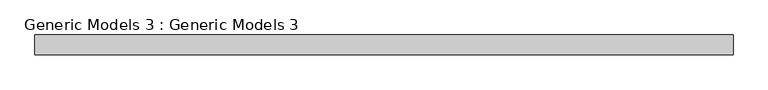
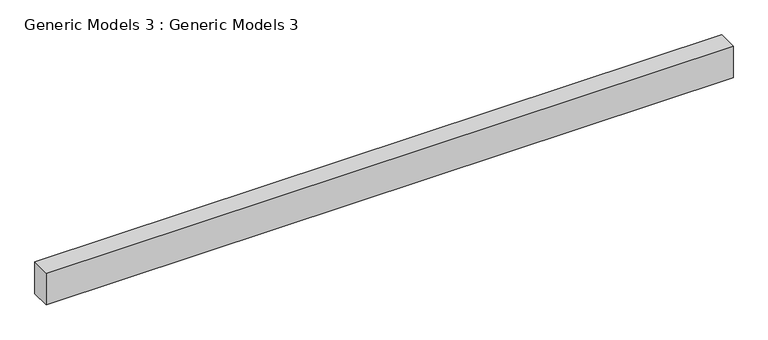
"""IFC4 building model written with IfcOpenShell, lengths in millimetres: proxy geometry, Generic Models 3 : Generic Models 3."""

from ifc_helpers import new_model, si_unit, frame, origin, place, context, project, spatial, polyline, outline, extrude, source, transform, mapped, element, save


def generic_models_3_generic_models_3_29ab51b9(model_context):
    return source(origin(), model_context, "Body", "SweptSolid", [
        extrude(outline(polyline([(3050.6885925, -21256.3670305), (-7701.088074, -21256.3670305), (-7701.088074, -20951.5670305), (3050.6885925, -20951.5670305), (3050.6885925, -21256.3670305)])), frame((0.0, 0.0, 29355.34491), z_axis=(0.0, 0.0, 1.0), x_axis=(1.0, 0.0, 0.0)), (0.0, 0.0, 1.0), 524.2840962),
    ])


if __name__ == "__main__":
    model = new_model("IFC4")
    model_context = context("Model", 3, world=origin())
    ifc_project = project(units=[si_unit("LENGTHUNIT", "METRE", prefix="MILLI")], contexts=[model_context])
    site = spatial("IfcSite", under=ifc_project)
    building = spatial("IfcBuilding", under=site)
    placement = place(None, origin())
    generic_models_3_generic_models_3_shape = generic_models_3_generic_models_3_29ab51b9(model_context)
    element("IfcBuildingElementProxy", 1, Name="Generic Models 3 : Generic Models 3", ObjectType="Generic Models 3 : Generic Models 3", at=placement, inside=building, context=model_context, shape_type="MappedRepresentation", body=[
        mapped(generic_models_3_generic_models_3_shape, transform((0.0, 0.0, 0.0), x_axis=(1.0, 0.0, 0.0), y_axis=(0.0, 1.0, 0.0), z_axis=(0.0, 0.0, 1.0))),
    ])
    save(model, "model.ifc")
